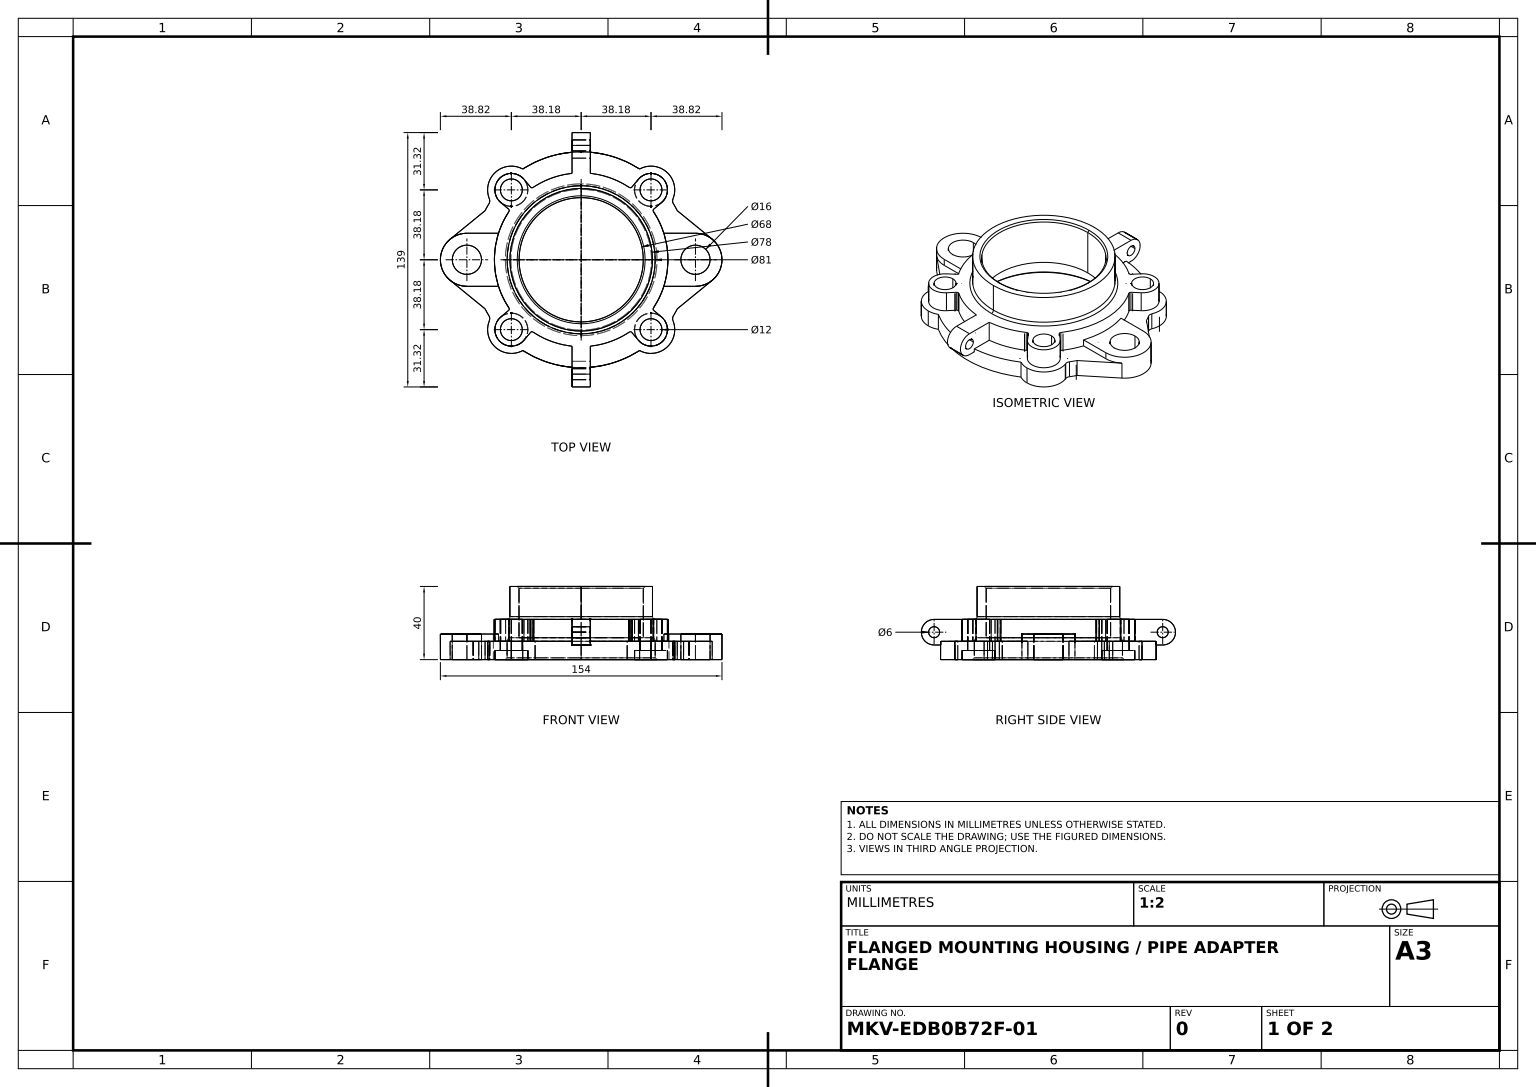
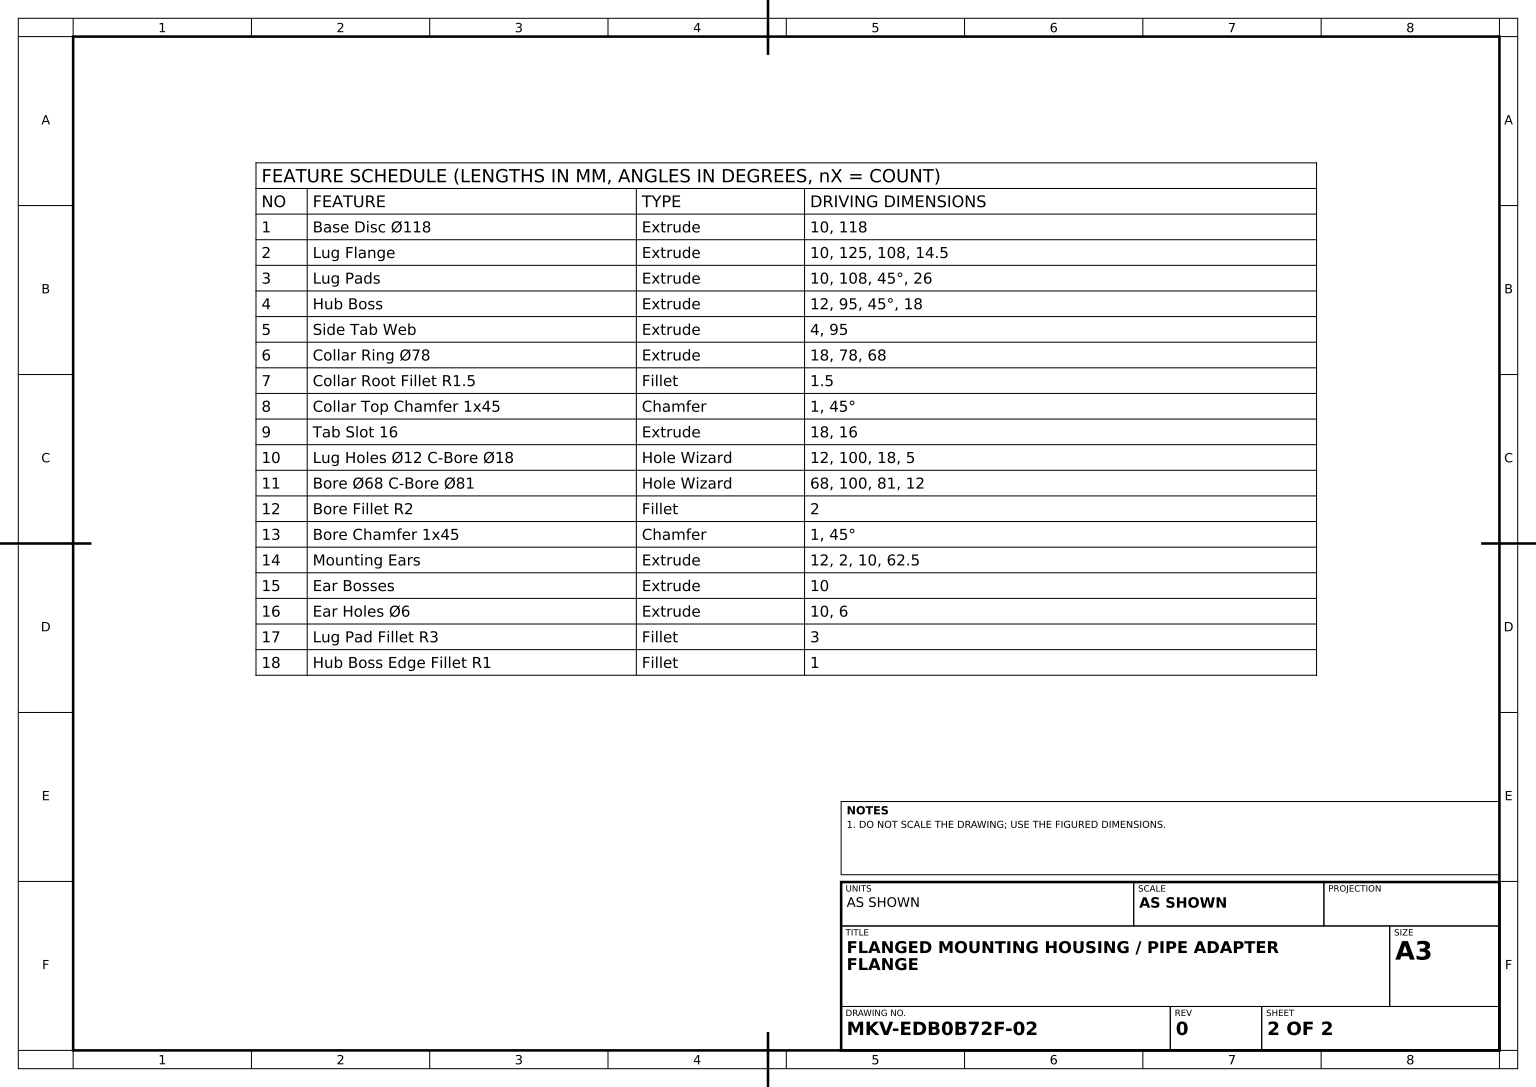
SolidWorks part; units mm, degrees
material "PE High Density"
ref_plane "Front Plane" through (0, 0, 0) normal (0, 0, 1) x (1, 0, 0)
ref_plane "Top Plane" through (0, 0, 0) normal (0, 1, 0) x (1, 0, 0)
ref_plane "Right Plane" through (0, 0, 0) normal (1, 0, 0) x (0, 0, -1)
sketch "Base Disc Sketch" plane through (0, 0, 0) normal (0, 1, 0) x (1, 0, 0)
  circle A0 centre (0, 0) radius 59
  dimension "D1" = 118
extrude "Base Disc Ø118" add sketch "Base Disc Sketch" along normal blind 10
sketch "Lug Flange Sketch" plane through (0, 0, 0) normal (0, -1, 0) x (1, 0, 0)
  line L0 (0, 0) -> (92.6281, 0) construction
  line L1 (0, 0) -> (0, -35.8161) construction
  line L2 (71.664, 11.237) -> (52.5488, 26.8258)
  line L3 (71.664, -11.237) -> (52.5488, -26.8258)
  line L4 (52.5488, 26.8258) -> (34.128, 41.8483) construction
  line L5 (52.5488, -26.8258) -> (34.128, -41.8483) construction
  line L6 (-52.5488, 26.8258) -> (-34.128, 41.8483) construction
  line L7 (-52.5488, -26.8258) -> (-34.128, -41.8483) construction
  line L8 (-71.664, -11.237) -> (-52.5488, -26.8258)
  line L9 (-71.664, 11.237) -> (-52.5488, 26.8258)
  circle A0 centre (0, 0) radius 62.5 construction
  circle A1 centre (0, 0) radius 54 construction
  arc A3 (71.664, -11.237) -> (71.664, 11.237) centre (62.5, 0) ccw
  circle A4 centre (0, 0) radius 59 construction
  arc A5 (52.5488, 26.8258) -> (-52.5488, 26.8258) centre (0, 0) ccw
  arc A6 (-71.664, -11.237) -> (-71.664, 11.237) centre (-62.5, 0) cw
  arc A7 (-52.5488, -26.8258) -> (52.5488, -26.8258) centre (0, 0) ccw
  dimension "D1" = 125
  dimension "D2" = 108
  dimension "D3" = 14.5
extrude "Lug Flange" add sketch "Lug Flange Sketch" against normal blind 10
sketch "Lug Pads Sketch" plane through (0, 10, 0) normal (0, 1, 0) x (1, 0, 0)
  line L0 (0, 0) -> (-73.9848, -73.9848) construction
  line L1 (0, 0) -> (-96.4964, 0) construction
  line L2 (0, 0) -> (0, 35.0843) construction
  circle A0 centre (0, 0) radius 54 construction
  arc A1 (-49.5957, -31.9573) -> (-31.9573, -49.5957) centre (-38.1838, -38.1838) ccw
  arc A2 (-49.5957, 31.9573) -> (-31.9573, 49.5957) centre (-38.1838, 38.1838) cw
  circle A3 centre (0, 0) radius 59
  arc A4 (-31.9573, -49.5957) -> (31.9573, -49.5957) centre (0, 0) ccw
  arc A5 (49.5957, -31.9573) -> (31.9573, -49.5957) centre (38.1838, -38.1838) cw
  arc A6 (49.5957, 31.9573) -> (31.9573, 49.5957) centre (38.1838, 38.1838) ccw
  arc A7 (-49.5957, 31.9573) -> (-49.5957, -31.9573) centre (0, 0) ccw
  arc A8 (31.9573, 49.5957) -> (-31.9573, 49.5957) centre (0, 0) ccw
  arc A9 (49.5957, -31.9573) -> (49.5957, 31.9573) centre (0, 0) ccw
  dimension "D1" = 108
  dimension "D3" = 26
  dimension "D2" = 45
  dimension "D4" = 0
extrude "Lug Pads" add sketch "Lug Pads Sketch" against normal blind 10
sketch "Hub Boss Sketch" plane through (0, 10, 0) normal (0, 1, 0) x (1, 0, 0)
  line L0 (0, 0) -> (-107.8408, 0) construction
  line L1 (0, 0) -> (-63.9625, 63.9625) construction
  line L2 (-31.3116, -43.9953) -> (-27.0978, -39.0123)
  line L3 (-43.9953, 31.3116) -> (-39.0123, 27.0978)
  line L4 (-31.3116, 43.9953) -> (-27.0978, 39.0123)
  line L5 (-43.9953, -31.3116) -> (-39.0123, -27.0978)
  line L6 (0, 0) -> (0, -13.7071) construction
  line L7 (31.3116, -43.9953) -> (27.0978, -39.0123)
  line L8 (43.9953, -31.3116) -> (39.0123, -27.0978)
  line L9 (31.3116, 43.9953) -> (27.0978, 39.0123)
  line L10 (43.9953, 31.3116) -> (39.0123, 27.0978)
  arc A0 (-39.0123, 27.0978) -> (-39.0123, -27.0978) centre (0, 0) ccw
  circle A1 centre (0, 0) radius 54 construction
  arc A2 (-31.3116, 43.9953) -> (-43.9953, 31.3116) centre (-38.1838, 38.1838) ccw
  arc A3 (-31.9573, 49.5957) -> (-49.5957, 31.9573) centre (-38.1838, 38.1838) ccw construction
  arc A5 (-31.3116, -43.9953) -> (-43.9953, -31.3116) centre (-38.1838, -38.1838) cw
  arc A6 (-27.0978, -39.0123) -> (27.0978, -39.0123) centre (0, 0) ccw
  arc A7 (31.3116, -43.9953) -> (43.9953, -31.3116) centre (38.1838, -38.1838) ccw
  arc A8 (31.3116, 43.9953) -> (43.9953, 31.3116) centre (38.1838, 38.1838) cw
  arc A9 (39.0123, -27.0978) -> (39.0123, 27.0978) centre (0, 0) ccw
  arc A10 (27.0978, 39.0123) -> (-27.0978, 39.0123) centre (0, 0) ccw
  dimension "D1" = 95
  dimension "D2" = 18
  dimension "D3" = 45
extrude "Hub Boss" add sketch "Hub Boss Sketch" along normal blind 12
sketch "Side Tab Sketch" plane through (0, 10, 0) normal (0, 1, 0) x (1, 0, 0)
  line L0 (-62.5, 14.5) -> (-45.2327, 14.5)
  line L1 (-62.5, -14.5) -> (-45.2327, -14.5)
  line L2 (0, 0) -> (0, 27.8375) construction
  line L3 (62.5, -14.5) -> (45.2327, -14.5)
  line L4 (62.5, 14.5) -> (45.2327, 14.5)
  arc A0 (-62.5, 14.5) -> (-62.5, -14.5) centre (-62.5, 0) ccw
  arc A1 (-71.664, 11.237) -> (-71.664, -11.237) centre (-62.5, 0) ccw construction
  arc A2 (-45.2327, -14.5) -> (45.2327, -14.5) centre (0, 0) ccw
  arc A3 (62.5, 14.5) -> (62.5, -14.5) centre (62.5, 0) cw
  arc A4 (45.2327, 14.5) -> (-45.2327, 14.5) centre (0, 0) ccw
  dimension "D1" = 95
extrude "Side Tab Web" add sketch "Side Tab Sketch" along normal blind 4
sketch "Collar Ring Sketch" plane through (0, 22, 0) normal (0, 1, 0) x (1, 0, 0)
  circle A0 centre (0, 0) radius 39
  arc A1 (27.0978, 39.0123) -> (-27.0978, 39.0123) centre (0, 0) ccw construction
  circle A2 centre (0, 0) radius 34
  dimension "D1" = 78
  dimension "D2" = 68
extrude "Collar Ring Ø78" add sketch "Collar Ring Sketch" along normal blind 18
fillet "Collar Root Fillet R1.5" radius 1.5 1 edges at (0, 22, -39)
chamfer "Collar Top Chamfer 1x45" distance 1 angle 45 1 edges at (0, 40, 34)
sketch "Tab Slot Sketch" plane through (0, 14, 0) normal (0, 1, 0) x (1, 0, 0)
  circle A0 centre (-62.5, 0) radius 8
  arc A1 (-62.5, 14.5) -> (-62.5, -14.5) centre (-62.5, 0) ccw construction
  circle A2 centre (62.5, 0) radius 8
  arc A3 (62.5, -14.5) -> (62.5, 14.5) centre (62.5, 0) ccw construction
  dimension "D1" = 16
extrude "Tab Slot 16" cut sketch "Tab Slot Sketch" against normal blind 18
hole_wizard "Lug Holes Ø12 C-Bore Ø18" positions "3DSketch1" profile "Sketch11" legacy
sketch3d "3DSketch1"
  arc A0 (-49.5957, 0, 31.9573) -> (-31.9573, 0, 49.5957) centre (-38.1838, 0, 38.1838) ccw construction
  arc A1 (31.9573, 0, 49.5957) -> (49.5957, 0, 31.9573) centre (38.1838, 0, 38.1838) ccw construction
  arc A2 (-31.9573, 0, -49.5957) -> (-49.5957, 0, -31.9573) centre (-38.1838, 0, -38.1838) ccw construction
  arc A3 (49.5957, 0, -31.9573) -> (31.9573, 0, -49.5957) centre (38.1838, 0, -38.1838) ccw construction
  point P0 (-38.1838, 0, 38.1838)
  point P2 (38.1838, 0, 38.1838)
  point P4 (38.1838, 0, -38.1838)
  point P6 (-38.1838, 0, -38.1838)
  point P13 (-38.1838, 13, 38.1838)
  point P18 (38.1838, 13, 38.1838)
  point P23 (-38.1838, 13, -38.1838)
  point P28 (38.1838, 13, -38.1838)
sketch "Sketch11" plane through (-38.1838, 0, 38.1838) normal (1, 0, 0) x (0, 0, -1)
  line L0 (0, 0) -> (0, 99.955)
  line L1 (0, 99.955) -> (6, 99.955)
  line L2 (6, 99.955) -> (6, 5)
  line L3 (6, 5) -> (9, 5)
  line L4 (9, 5) -> (9, 0)
  line L5 (9, 0) -> (0, 0)
  line L6 (0, 110) -> (0, -10) construction
  dimension "Diameter" = 12
  dimension "Depth" = 100
  dimension "C-Bore Diameter" = 18
  dimension "C-Bore Depth" = 5
hole_wizard "Bore Ø68 C-Bore Ø81" positions "3DSketch2" profile "Sketch13" legacy
sketch3d "3DSketch2"
  arc A0 (-31.9573, 0, 49.5957) -> (31.9573, 0, 49.5957) centre (0, 0, 0) ccw construction
  point P0 (0, 0, 0)
  point P3 (0, 0, 0)
  point P9 (0, 59, 0)
sketch "Sketch13" plane through (0, 0, 0) normal (1, 0, 0) x (0, 0, -1)
  line L0 (0, 0) -> (0, 99.7885)
  line L1 (0, 99.7885) -> (34, 99.7885)
  line L2 (34, 99.7885) -> (34, 12)
  line L3 (34, 12) -> (40.5, 12)
  line L4 (40.5, 12) -> (40.5, 0)
  line L5 (40.5, 0) -> (0, 0)
  line L6 (0, 110) -> (0, -10) construction
  dimension "Diameter" = 68
  dimension "Depth" = 100
  dimension "C-Bore Diameter" = 81
  dimension "C-Bore Depth" = 12
fillet "Bore Fillet R2" radius 2 1 edges at (0, 12, -40.5)
chamfer "Bore Chamfer 1x45" distance 1 angle 45 1 edges at (0, 0, -40.5)
sketch "Mounting Ear Sketch" plane through (0, 10, 0) normal (0, 1, 0) x (1, 0, 0)
  line L0 (0, 0) -> (-107.7581, 0) construction
  line L1 (-5, 47.2361) -> (5, 47.2361)
  line L2 (-5, 47.2361) -> (-5, 62.5)
  line L3 (-5, 62.5) -> (5, 62.5)
  line L4 (5, 47.2361) -> (5, 62.5)
  line L5 (-5, -47.2361) -> (5, -47.2361)
  line L6 (-5, -62.5) -> (5, -62.5)
  line L7 (5, -47.2361) -> (5, -62.5)
  line L8 (-5, -47.2361) -> (-5, -62.5)
  arc A0 (27.0978, 39.0123) -> (-27.0978, 39.0123) centre (0, 0) ccw construction
  point P4 (0, 47.2361)
  dimension "D1" = 10
  dimension "D2" = 62.5
extrude "Mounting Ears" add sketch "Mounting Ear Sketch" along normal blind 12 and the other way blind 2
sketch "Ear Boss Sketch" plane through (5, 0, 0) normal (1, 0, 0) x (0, 0, -1)
  line L0 (62.5, 8) -> (62.5, 22) construction
  line L1 (-62.5, 8) -> (-62.5, 22) construction
  line L2 (-62.5, 22) -> (-47.2361, 22) construction
  circle A0 centre (62.5, 15) radius 7
  circle A1 centre (-62.5, 15) radius 7
extrude "Ear Bosses" add sketch "Ear Boss Sketch" against normal blind 10
sketch "Ear Hole Sketch" plane through (5, 0, 0) normal (1, 0, 0) x (0, 0, -1)
  circle A0 centre (-62.5, 15) radius 3
  arc A1 (-62.5, 22) -> (-62.5, 8) centre (-62.5, 15) ccw construction
  circle A2 centre (62.5, 15) radius 3
  arc A3 (62.5, 8) -> (62.5, 22) centre (62.5, 15) ccw construction
  dimension "D1" = 6
extrude "Ear Holes Ø6" cut sketch "Ear Hole Sketch" against normal blind 10
fillet "Lug Pad Fillet R3" radius 3 4 edges at (-49.5957, 5, -31.9573) (49.5957, 5, -31.9573) (49.5957, 5, 31.9573) (-49.5957, 5, 31.9573)
fillet "Hub Boss Edge Fillet R1" radius 1 8 edges at (-27.0978, 16, 39.0123) (-39.0123, 16, 27.0978) (-39.0123, 16, -27.0978) (-27.0978, 16, -39.0123) (27.0978, 16, -39.0123) (39.0123, 16, -27.0978) (39.0123, 16, 27.0978) (27.0978, 16, 39.0123)
